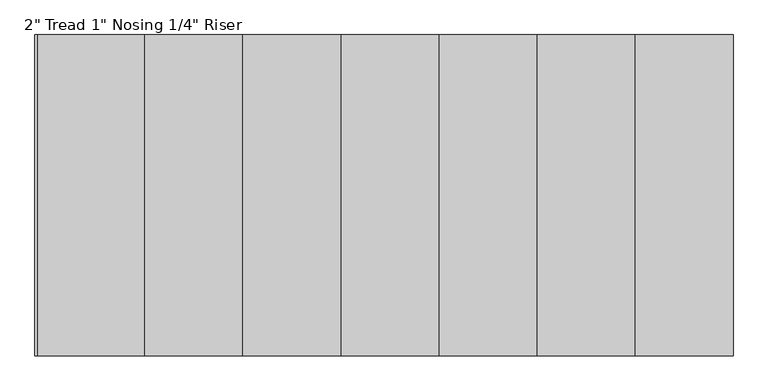
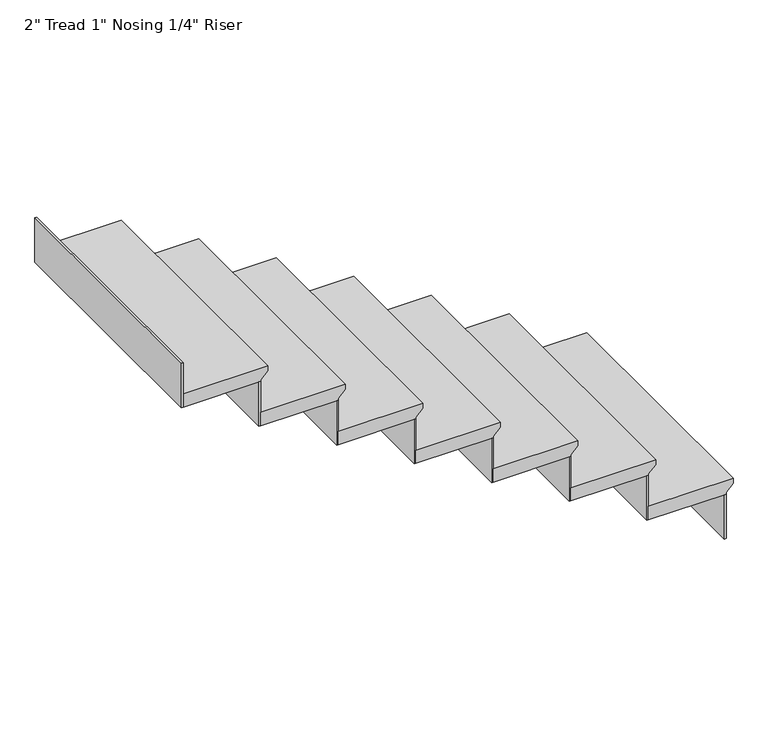
"""IFC4 building model written with IfcOpenShell, lengths in millimetres: stair flight geometry."""

from ifc_helpers import new_model, si_unit, frame, origin, place, context, project, spatial, polyline, outline, extrude, source, transform, mapped, element, save


def stair_flight_5d59741f(model_context):
    return source(origin(), model_context, "Body", "SweptSolid", [
        extrude(outline(polyline([(1676.4, 678.235938), (1676.4, 373.435938), (1625.6, 373.435938), (1625.6, 652.835938), (1631.95, 652.835938), (1657.35, 678.235938), (1676.4, 678.235938)])), frame((0.0, 1120.5857363, 0.0), z_axis=(0.0, 1.0, 0.0), x_axis=(0.0, 0.0, 1.0)), (0.0, 0.0, 1.0), 914.4),
        extrude(outline(polyline([(646.485938, 2034.9857363), (652.835938, 2034.9857363), (652.835938, 1120.5857363), (646.485938, 1120.5857363), (646.485938, 2034.9857363)])), frame((0.0, 0.0, 1456.2666667), z_axis=(0.0, 0.0, 1.0), x_axis=(1.0, 0.0, 0.0)), (0.0, 0.0, 1.0), 169.3333333),
        extrude(outline(polyline([(367.085938, 2034.9857363), (373.435938, 2034.9857363), (373.435938, 1120.5857363), (367.085938, 1120.5857363), (367.085938, 2034.9857363)])), frame((0.0, 0.0, 1625.6), z_axis=(0.0, 0.0, 1.0), x_axis=(1.0, 0.0, 0.0)), (0.0, 0.0, 1.0), 169.3333333),
        extrude(outline(polyline([(1845.7333333, 398.835938), (1845.7333333, 94.035938), (1794.9333333, 94.035938), (1794.9333333, 373.435938), (1801.2833333, 373.435938), (1826.6833333, 398.835938), (1845.7333333, 398.835938)])), frame((0.0, 1120.5857363, 0.0), z_axis=(0.0, 1.0, 0.0), x_axis=(0.0, 0.0, 1.0)), (0.0, 0.0, 1.0), 914.4),
        extrude(outline(polyline([(87.685938, 2034.9857363), (94.035938, 2034.9857363), (94.035938, 1120.5857363), (87.685938, 1120.5857363), (87.685938, 2034.9857363)])), frame((0.0, 0.0, 1794.9333333), z_axis=(0.0, 0.0, 1.0), x_axis=(1.0, 0.0, 0.0)), (0.0, 0.0, 1.0), 169.3333333),
        extrude(outline(polyline([(2015.0666667, 119.435938), (2015.0666667, -185.364062), (1964.2666667, -185.364062), (1964.2666667, 94.035938), (1970.6166667, 94.035938), (1996.0166667, 119.435938), (2015.0666667, 119.435938)])), frame((0.0, 1120.5857363, 0.0), z_axis=(0.0, 1.0, 0.0), x_axis=(0.0, 0.0, 1.0)), (0.0, 0.0, 1.0), 914.4),
        extrude(outline(polyline([(-191.714062, 2034.9857363), (-185.364062, 2034.9857363), (-185.364062, 1120.5857363), (-191.714062, 1120.5857363), (-191.714062, 2034.9857363)])), frame((0.0, 0.0, 1964.2666667), z_axis=(0.0, 0.0, 1.0), x_axis=(1.0, 0.0, 0.0)), (0.0, 0.0, 1.0), 169.3333333),
        extrude(outline(polyline([(2184.4, -159.964062), (2184.4, -464.764062), (2133.6, -464.764062), (2133.6, -185.364062), (2139.95, -185.364062), (2165.35, -159.964062), (2184.4, -159.964062)])), frame((0.0, 1120.5857363, 0.0), z_axis=(0.0, 1.0, 0.0), x_axis=(0.0, 0.0, 1.0)), (0.0, 0.0, 1.0), 914.4),
        extrude(outline(polyline([(-471.114062, 2034.9857363), (-464.764062, 2034.9857363), (-464.764062, 1120.5857363), (-471.114062, 1120.5857363), (-471.114062, 2034.9857363)])), frame((0.0, 0.0, 2133.6), z_axis=(0.0, 0.0, 1.0), x_axis=(1.0, 0.0, 0.0)), (0.0, 0.0, 1.0), 169.3333333),
        extrude(outline(polyline([(2353.7333333, -439.364062), (2353.7333333, -744.164062), (2302.9333333, -744.164062), (2302.9333333, -464.764062), (2309.2833333, -464.764062), (2334.6833333, -439.364062), (2353.7333333, -439.364062)])), frame((0.0, 1120.5857363, 0.0), z_axis=(0.0, 1.0, 0.0), x_axis=(0.0, 0.0, 1.0)), (0.0, 0.0, 1.0), 914.4),
        extrude(outline(polyline([(-750.514062, 2034.9857363), (-744.164062, 2034.9857363), (-744.164062, 1120.5857363), (-750.514062, 1120.5857363), (-750.514062, 2034.9857363)])), frame((0.0, 0.0, 2302.9333333), z_axis=(0.0, 0.0, 1.0), x_axis=(1.0, 0.0, 0.0)), (0.0, 0.0, 1.0), 169.3333333),
        extrude(outline(polyline([(2523.0666667, -718.764062), (2523.0666667, -1023.564062), (2472.2666667, -1023.564062), (2472.2666667, -744.164062), (2478.6166667, -744.164062), (2504.0166667, -718.764062), (2523.0666667, -718.764062)])), frame((0.0, 1120.5857363, 0.0), z_axis=(0.0, 1.0, 0.0), x_axis=(0.0, 0.0, 1.0)), (0.0, 0.0, 1.0), 914.4),
        extrude(outline(polyline([(-1029.914062, 2034.9857363), (-1023.564062, 2034.9857363), (-1023.564062, 1120.5857363), (-1029.914062, 1120.5857363), (-1029.914062, 2034.9857363)])), frame((0.0, 0.0, 2472.2666667), z_axis=(0.0, 0.0, 1.0), x_axis=(1.0, 0.0, 0.0)), (0.0, 0.0, 1.0), 169.3333333),
        extrude(outline(polyline([(-1309.314062, 2034.9857363), (-1302.964062, 2034.9857363), (-1302.964062, 1120.5857363), (-1309.314062, 1120.5857363), (-1309.314062, 2034.9857363)])), frame((0.0, 0.0, 2641.6), z_axis=(0.0, 0.0, 1.0), x_axis=(1.0, 0.0, 0.0)), (0.0, 0.0, 1.0), 169.3333333),
        extrude(outline(polyline([(2692.4, -998.164062), (2692.4, -1302.964062), (2641.6, -1302.964062), (2641.6, -1023.564062), (2647.95, -1023.564062), (2673.35, -998.164062), (2692.4, -998.164062)])), frame((0.0, 1120.5857363, 0.0), z_axis=(0.0, 1.0, 0.0), x_axis=(0.0, 0.0, 1.0)), (0.0, 0.0, 1.0), 914.4),
    ])


if __name__ == "__main__":
    model = new_model("IFC4")
    model_context = context("Model", 3, world=origin())
    ifc_project = project(units=[si_unit("LENGTHUNIT", "METRE", prefix="MILLI")], contexts=[model_context])
    site = spatial("IfcSite", under=ifc_project)
    building = spatial("IfcBuilding", under=site)
    placement = place(None, origin())
    stair_flight_shape = stair_flight_5d59741f(model_context)
    element("IfcStairFlight", 1, ObjectType="2\" Tread 1\" Nosing 1/4\" Riser", at=placement, inside=building, context=model_context, shape_type="MappedRepresentation", body=[
        mapped(stair_flight_shape, transform((0.0, 0.0, 0.0), x_axis=(1.0, 0.0, 0.0), y_axis=(0.0, 1.0, 0.0), z_axis=(0.0, 0.0, 1.0))),
    ])
    save(model, "model.ifc")

# Revit data of these elements
# Element 1 (IfcStairFlight, "2\" Tread 1\" Nosing 1/4\" Riser")
#   Materials on its faces: "BURGUNDY COLOUR"
# Materials
#   "BURGUNDY COLOUR": class "Generic", colour RGB 120 120 120, transparency 0, Cost = 0
